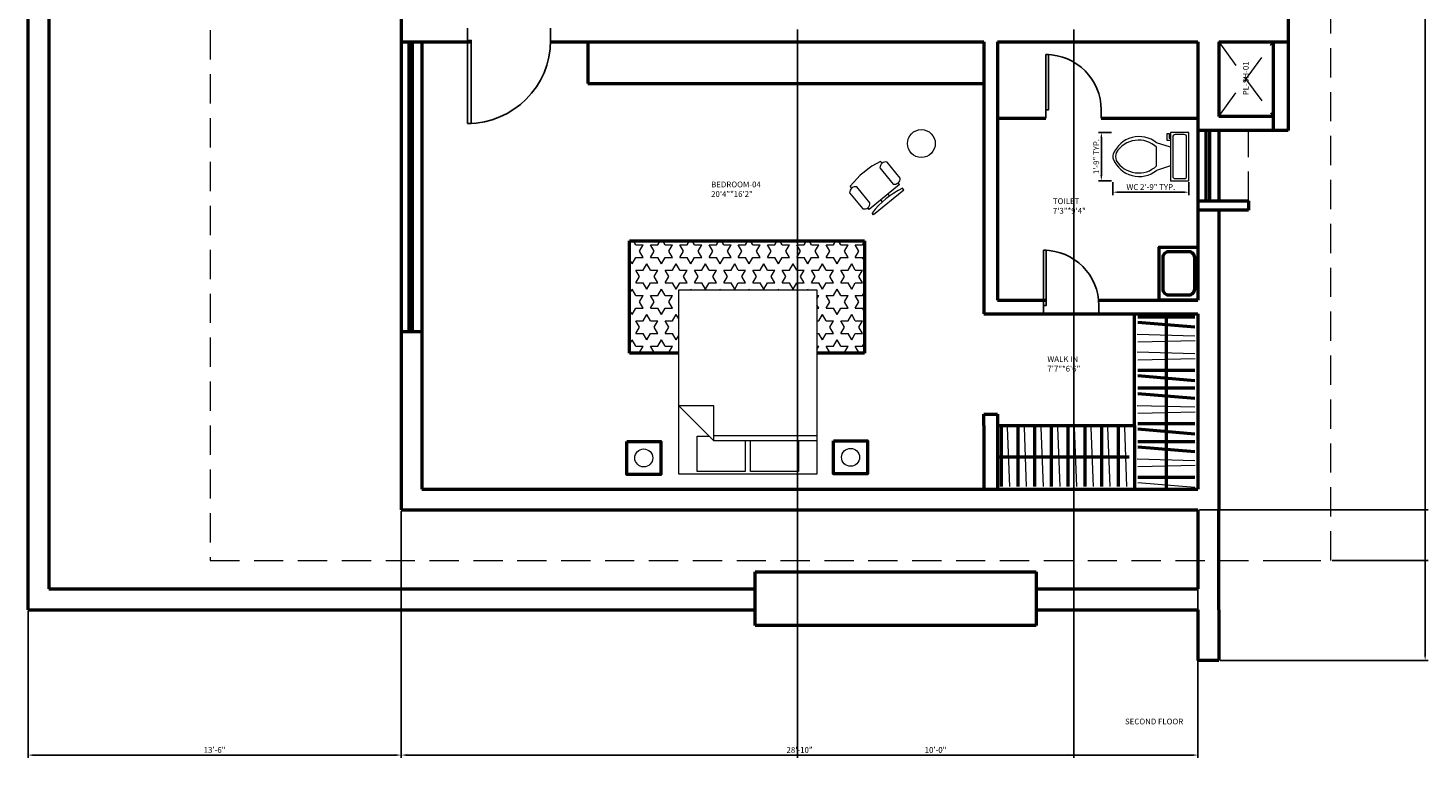
# Model space of a CAD drawing. Units: inches. Extents: x 5312 to 23584, y 2846 to 7447.
# Tile 7 of 12: x 10692 to 11300, y 3035 to 3352. Entities that reach past the tile are written whole.
import ezdxf

# ---------------------------------------------------------------- set-up
doc = ezdxf.new("R2010")
doc.units = ezdxf.units.IN
doc.linetypes.add('DASHED', pattern=[19.05, 12.7, -6.35])
for name, color, linetype, lineweight in [('A-ANNO-DIMS', 2, 'Continuous', 18), ('A-ANNO-TEXT', 3, 'Continuous', 18), ('A-AREA-IDEN', 7, 'Continuous', 18), ('A-DOOR', 4, 'Continuous', 25), ('A-FLOR-FIXT', 9, 'Continuous', 18), ('A-FLOR-OVHD', 8, 'DASHED', 18), ('A-FLOR-PATT', 252, 'Continuous', 13), ('A-FURN', 8, 'Continuous', 18), ('A-WALL', 7, 'Continuous', 50)]:
    doc.layers.add(name, color=color, linetype=linetype, lineweight=lineweight)
doc.styles.get("Standard").update_dxf_attribs({"font": 'arial.ttf'})
doc.dimstyles.new('ISO-25', dxfattribs={"dimtxt": 2.5, "dimasz": 2.5, "dimexe": 1.25, "dimexo": 0.625, "dimtad": 1, "dimlunit": 3, "dimtxsty": 'Standard', "dimcen": 2.5, "dimadec": 0, "dimazin": 0, "dimtfac": 1, "dimtmove": 0, "dimatfit": 3, "dimfxl": 1, "dimarcsym": 0})

# ---------------------------------------------------------------- blocks, each defined once
blk = doc.blocks.new('*U2')
for p, q in [((0, 0), (0, -6)), ((40, 0), (40, -6))]:
    blk.add_line(p, q)
blk.add_lwpolyline([(0, 0), (0, 40), (1.75, 40), (1.75, 0)], close=True)
blk.add_arc((0, 0), 40, 0, 90)
blk = doc.blocks.new('Toilet - top')
for p, q in [((9.5, -6), (9.5, -2)), ((-10, -8.5), (-8, -8.5)), ((-10, -9.5), (-10, -8.5)), ((-7, -9.5), (-10, -9.5)), ((-8, -8.5), (-8, -8)), ((-7, -8), (-7, -9.5)), ((-4, -8), (-6, -14)), ((4, -8), (6, -14)), ((4, -14), (-4, -14))]:
    blk.add_line(p, q)
blk.add_lwpolyline([(10.5, -8), (10.5, 0), (-10.5, 0), (-10.5, -8)], close=True)
for points in [[(-9.5, -2), (-9.5, -6)], [(8.5, -1), (-8.5, -1)], [(-8.5, -7), (8.5, -7)]]:
    blk.add_lwpolyline(points)
for centre, radius, start, end in [((-8.62, -1.88), 0.884, 81.8699, 188.1301), ((-8.62, -6.12), 0.884, 171.8699, 278.1301), ((8.62, -1.88), 0.884, 351.8699, 98.1301), ((8.62, -6.12), 0.884, 261.8699, 8.1301), ((3.52, -21.58), 12.17, 141.46911, 247.97143), ((4.2, -21.82), 11.33, 136.36773, 238.94682), ((-3.52, -21.58), 12.17, 292.02843, 38.53071), ((-4.2, -21.82), 11.33, 301.05301, 43.63209), ((0, -27.88), 4, 245.73182, 294.26817), ((0, -29), 4, 254.86053, 285.13947)]:
    blk.add_arc(centre, radius, start, end)
blk = doc.blocks.new('Bed - Queen')
for p, q in [((0, -80.00003), (0, 0)), ((0, 0), (59.99999, 0)), ((59.99999, 0), (59.99999, -80.00003)), ((7.99999, -1.2), (28.79998, -1.2)), ((7.99999, -14.4), (7.99999, -1.2)), ((28.79998, -1.2), (28.79998, -14.4)), ((31.19999, -1.2), (51.99999, -1.2)), ((31.19999, -14.4), (31.19999, -1.2)), ((51.99999, -1.2), (51.99999, -16.4)), ((0, -14.4), (44.8, -14.4)), ((44.8, -16.8), (0, -16.8)), ((59.99999, -29.6), (44.8, -14.4)), ((44.8, -14.4), (44.8, -29.6)), ((51.99999, -16.4), (46.79936, -16.4)), ((44.8, -29.6), (59.99999, -29.6)), ((59.99999, -80.00003), (0, -80.00003))]:
    blk.add_line(p, q)
blk = doc.blocks.new('Chair - Desk')
for p, q in [((-8.5, 0), (-8.5, -1)), ((-8.5, 0), (8.5, 0)), ((8.5, 0), (8.5, -1)), ((-10.5, -5), (-10.5, -14)), ((-8.5, -3), (-8.5, -4)), ((-8.5, -3), (8.5, -3)), ((-6.5, -14), (-6.5, -5)), ((-2, -3), (-2, -1.9355)), ((2, -1.9576), (2, -3)), ((6.5, -5), (6.5, -14)), ((8.5, -3), (8.5, -4)), ((10.5, -14), (10.5, -5)), ((-8.5, -15), (-8.5, -16)), ((8.5, -15), (8.5, -16))]:
    blk.add_line(p, q)
for centre, radius, start, end in [((-8.5, -6.5), 2.5, 36.8699, 143.1301), ((0, 34.625), 36.625, 256.5803, 283.4197), ((8.5, -6.5), 2.5, 36.8699, 143.1301), ((-8.5, -12.5), 2.5, 216.8699, 323.1301), ((0, 19.625), 36.625, 256.5803, 283.4197), ((8.5, -12.5), 2.5, 216.8699, 323.1301)]:
    blk.add_arc(centre, radius, start, end)
blk = doc.blocks.new('WARDROBE-HANGER')
for p, q in [((0, 3.4), (24.8, 3.4)), ((0, 1.32), (24.99, 0))]:
    blk.add_line(p, q)
blk = doc.blocks.new('*D29')
at = {"layer": 'A-ANNO-DIMS', "color": 0, "lineweight": -2, "transparency": 16777216}
for p, q in [((11162.96, 3285.09), (11162.96, 3279.51)), ((11196.01, 3285.09), (11196.01, 3279.51)), ((11165.46, 3280.76), (11193.51, 3280.76))]:
    blk.add_line(p, q, dxfattribs=at)
at = {"layer": 'A-ANNO-DIMS', "color": 0, "transparency": 16777216}
for points in [[(11165.46, 3281.18), (11165.46, 3280.34), (11162.96, 3280.76)], [(11193.51, 3281.18), (11193.51, 3280.34), (11196.01, 3280.76)]]:
    blk.add_solid(points, dxfattribs=at)
at = {"layer": 'DEFPOINTS', "color": 0, "transparency": 16777216}
for p in [(11162.96, 3285.72), (11196.01, 3285.72), (11196.01, 3280.76)]:
    blk.add_point(p, dxfattribs=at)
at = {"layer": 'A-ANNO-DIMS', "color": 0, "transparency": 16777216, "insert": (11179.49, 3282.68), "char_height": 2.5, "attachment_point": 5}
blk.add_mtext('WC 2\'-9" TYP.', dxfattribs=at)
blk = doc.blocks.new('*D30')
at = {"layer": 'A-ANNO-DIMS', "color": 0, "lineweight": -2, "transparency": 16777216}
for p, q in [((11162.34, 3306.72), (11156.76, 3306.72)), ((11158.01, 3304.22), (11158.01, 3288.22)), ((11162.34, 3285.72), (11156.76, 3285.72))]:
    blk.add_line(p, q, dxfattribs=at)
at = {"layer": 'A-ANNO-DIMS', "color": 0, "transparency": 16777216}
for points in [[(11157.59, 3304.22), (11158.42, 3304.22), (11158.01, 3306.72)], [(11157.59, 3288.22), (11158.42, 3288.22), (11158.01, 3285.72)]]:
    blk.add_solid(points, dxfattribs=at)
at = {"layer": 'DEFPOINTS', "color": 0, "transparency": 16777216}
for p in [(11162.96, 3306.72), (11158.01, 3285.72), (11162.96, 3285.72)]:
    blk.add_point(p, dxfattribs=at)
at = {"layer": 'A-ANNO-DIMS', "color": 0, "transparency": 16777216, "insert": (11156.1, 3296.22), "char_height": 2.5, "attachment_point": 5, "rotation": 90}
blk.add_mtext('1\'-9" TYP.', dxfattribs=at)
blk = doc.blocks.new('*D84')
at = {"layer": 'A-ANNO-DIMS', "color": 0, "lineweight": -2, "transparency": 16777216}
for p, q in [((11209.58, 3832.48), (11299.83, 3832.48)), ((11298.58, 3829.98), (11298.58, 3080.08)), ((11209.58, 3077.58), (11299.83, 3077.58))]:
    blk.add_line(p, q, dxfattribs=at)
at = {"layer": 'A-ANNO-DIMS', "color": 0, "transparency": 16777216}
for points in [[(11298.16, 3829.98), (11298.99, 3829.98), (11298.58, 3832.48)], [(11298.16, 3080.08), (11298.99, 3080.08), (11298.58, 3077.58)]]:
    blk.add_solid(points, dxfattribs=at)
at = {"layer": 'DEFPOINTS', "color": 0, "transparency": 16777216}
for p in [(11208.96, 3832.48), (11208.96, 3077.58), (11298.58, 3077.58)]:
    blk.add_point(p, dxfattribs=at)
at = {"layer": 'A-ANNO-DIMS', "color": 0, "transparency": 16777216, "insert": (11296.68, 3455.03), "char_height": 2.5, "attachment_point": 5, "rotation": 90}
blk.add_mtext('62\'-11"', dxfattribs=at)
blk = doc.blocks.new('*D89')
at = {"layer": 'A-ANNO-DIMS', "color": 0, "lineweight": -2, "transparency": 16777216}
for p, q in [((10853.96, 3142.35), (10853.96, 3035.33)), ((11199.96, 3142.35), (11199.96, 3035.33)), ((10856.46, 3036.58), (11197.46, 3036.58))]:
    blk.add_line(p, q, dxfattribs=at)
at = {"layer": 'A-ANNO-DIMS', "color": 0, "transparency": 16777216}
for points in [[(10856.46, 3037), (10856.46, 3036.17), (10853.96, 3036.58)], [(11197.46, 3037), (11197.46, 3036.17), (11199.96, 3036.58)]]:
    blk.add_solid(points, dxfattribs=at)
at = {"layer": 'DEFPOINTS', "color": 0, "transparency": 16777216}
for p in [(10853.96, 3142.97), (11199.96, 3142.97), (11199.96, 3036.58)]:
    blk.add_point(p, dxfattribs=at)
at = {"layer": 'A-ANNO-DIMS', "color": 0, "transparency": 16777216, "insert": (11026.96, 3038.48), "char_height": 2.5, "attachment_point": 5}
blk.add_mtext('28\'-10"', dxfattribs=at)
blk = doc.blocks.new('*D90')
at = {"layer": 'A-ANNO-DIMS', "color": 0, "lineweight": -2, "transparency": 16777216}
for p, q in [((10853.96, 3142.35), (10853.96, 3035.33)), ((10691.96, 3099.01), (10691.96, 3035.33)), ((10694.46, 3036.58), (10851.46, 3036.58))]:
    blk.add_line(p, q, dxfattribs=at)
at = {"layer": 'A-ANNO-DIMS', "color": 0, "transparency": 16777216}
for points in [[(10694.46, 3037), (10694.46, 3036.17), (10691.96, 3036.58)], [(10851.46, 3037), (10851.46, 3036.17), (10853.96, 3036.58)]]:
    blk.add_solid(points, dxfattribs=at)
at = {"layer": 'DEFPOINTS', "color": 0, "transparency": 16777216}
for p in [(10853.96, 3142.97), (10691.96, 3099.64), (10853.96, 3036.58)]:
    blk.add_point(p, dxfattribs=at)
at = {"layer": 'A-ANNO-DIMS', "color": 0, "transparency": 16777216, "insert": (10772.96, 3038.49), "char_height": 2.5, "attachment_point": 5}
blk.add_mtext('13\'-6"', dxfattribs=at)
blk = doc.blocks.new('*D91')
at = {"layer": 'A-ANNO-DIMS', "color": 0, "lineweight": -2, "transparency": 16777216}
for p, q in [((11200.58, 3706.97), (11299.83, 3706.97)), ((11298.58, 3704.47), (11298.58, 3145.47)), ((11200.58, 3142.97), (11299.83, 3142.97))]:
    blk.add_line(p, q, dxfattribs=at)
at = {"layer": 'A-ANNO-DIMS', "color": 0, "transparency": 16777216}
for points in [[(11298.16, 3704.47), (11298.99, 3704.47), (11298.58, 3706.97)], [(11298.16, 3145.47), (11298.99, 3145.47), (11298.58, 3142.97)]]:
    blk.add_solid(points, dxfattribs=at)
at = {"layer": 'DEFPOINTS', "color": 0, "transparency": 16777216}
for p in [(11199.96, 3706.97), (11199.96, 3142.97), (11298.58, 3142.97)]:
    blk.add_point(p, dxfattribs=at)
at = {"layer": 'A-ANNO-DIMS', "color": 0, "transparency": 16777216, "insert": (11296.68, 3424.97), "char_height": 2.5, "attachment_point": 5, "rotation": 90}
blk.add_mtext('47\'-0"', dxfattribs=at)
blk = doc.blocks.new('*D95')
at = {"layer": 'A-ANNO-DIMS', "color": 0, "lineweight": -2, "transparency": 16777216}
for p, q in [((11258.2, 3751.07), (11299.83, 3751.07)), ((11298.58, 3748.57), (11298.58, 3123.52)), ((11258.2, 3121.02), (11299.83, 3121.02))]:
    blk.add_line(p, q, dxfattribs=at)
at = {"layer": 'A-ANNO-DIMS', "color": 0, "transparency": 16777216}
for points in [[(11298.16, 3748.57), (11298.99, 3748.57), (11298.58, 3751.07)], [(11298.16, 3123.52), (11298.99, 3123.52), (11298.58, 3121.02)]]:
    blk.add_solid(points, dxfattribs=at)
at = {"layer": 'DEFPOINTS', "color": 0, "transparency": 16777216}
for p in [(11257.58, 3751.07), (11257.58, 3121.02), (11298.58, 3121.02)]:
    blk.add_point(p, dxfattribs=at)
at = {"layer": 'A-ANNO-DIMS', "color": 0, "transparency": 16777216, "insert": (11296.68, 3436.04), "char_height": 2.5, "attachment_point": 5, "rotation": 90}
blk.add_mtext('52\'-6"', dxfattribs=at)
blk = doc.blocks.new('*D97')
at = {"layer": 'A-ANNO-DIMS', "color": 0, "lineweight": -2, "transparency": 16777216}
for p, q in [((11026, 3351.35), (11026, 3035.33)), ((11146, 3351.35), (11146, 3035.33)), ((11028.5, 3036.58), (11143.5, 3036.58))]:
    blk.add_line(p, q, dxfattribs=at)
at = {"layer": 'A-ANNO-DIMS', "color": 0, "transparency": 16777216}
for points in [[(11028.5, 3037), (11028.5, 3036.17), (11026, 3036.58)], [(11143.5, 3037), (11143.5, 3036.17), (11146, 3036.58)]]:
    blk.add_solid(points, dxfattribs=at)
at = {"layer": 'DEFPOINTS', "color": 0, "transparency": 16777216}
for p in [(11026, 3351.97), (11146, 3351.97), (11146, 3036.58)]:
    blk.add_point(p, dxfattribs=at)
at = {"layer": 'A-ANNO-DIMS', "color": 0, "transparency": 16777216, "insert": (11086, 3038.48), "char_height": 2.5, "attachment_point": 5}
blk.add_mtext('10\'-0"', dxfattribs=at)

msp = doc.modelspace()

# ---------------------------------------------------------------- hatches: boundary and pattern name
at = {"layer": 'A-FLOR-PATT'}
h = msp.add_hatch(dxfattribs=at)
h.set_pattern_fill('STARS', color=256)
h.set_pattern_definition([(0, (27.571, -223.0893), (0, 5.4992613), [3.175, -3.175]), (60, (27.571, -223.0893), (-4.7625, 2.7496307), [3.175, -3.175]), (120, (29.1586, -220.3397), (-4.7625, -2.7496307), [3.175, -3.175])])
h.paths.add_polyline_path([(11055.106, 3259.675), (10953.169, 3259.675), (10953.169, 3210.954), (10974.489, 3210.954), (10974.489, 3238.461), (11034.489, 3238.461), (11034.489, 3210.954), (11055.106, 3210.954)])

# ---------------------------------------------------------------- linework, layer by layer
at = {"layer": 'A-FLOR-OVHD'}
for p, q in [((10771.06, 3751.067), (10771.06, 3121.017)), ((11257.577, 3121.017), (11257.577, 3751.067)), ((11208.956, 3345.971), (11232.596, 3313.569)), ((11208.956, 3313.569), (11232.596, 3345.971)), ((11221.852, 3276.968), (11221.852, 3307.569)), ((10771.06, 3121.017), (11240.609, 3121.017)), ((11240.609, 3121.017), (11257.577, 3121.017))]:
    msp.add_line(p, q, dxfattribs=at)
at = {"layer": 'A-FURN'}
for p, q in [((11117.157, 3178.678), (11118.144, 3153.125)), ((11124.419, 3178.678), (11125.405, 3153.125)), ((11131.68, 3178.678), (11132.666, 3153.125)), ((11138.941, 3178.678), (11139.927, 3153.125)), ((11146.203, 3178.678), (11147.189, 3153.125)), ((11153.464, 3178.678), (11154.45, 3153.125)), ((11160.725, 3178.678), (11161.711, 3153.125)), ((11167.987, 3178.678), (11168.973, 3153.125)), ((11173.853, 3154.871), (11198.546, 3152.788))]:
    msp.add_line(p, q, dxfattribs=at)
for centre, radius in [((11079.861, 3301.87), 6.038), ((10959.33, 3165.472), 3.898), ((11049.101, 3165.75), 3.898)]:
    msp.add_circle(centre, radius, dxfattribs=at)
at = {"layer": 'A-WALL'}
for p, q in [((10700.956, 3790.971), (10700.956, 3108.64)), ((10853.956, 3706.971), (10853.956, 3142.971)), ((11239.069, 3394.056), (11239.069, 3307.569)), ((10691.956, 3375.201), (10691.956, 3099.64)), ((10853.956, 3345.971), (10884.418, 3345.971)), ((10857.312, 3345.971), (10857.312, 3220.265)), ((10858.699, 3345.971), (10858.699, 3345.971)), ((10858.699, 3345.971), (10858.699, 3220.265)), ((10862.956, 3345.971), (10862.956, 3151.971)), ((10918.838, 3345.971), (11106.956, 3345.971)), ((10934.962, 3345.971), (10934.962, 3327.899)), ((11106.956, 3345.971), (11106.956, 3227.971)), ((11112.956, 3345.971), (11112.956, 3233.971)), ((11112.956, 3345.971), (11199.956, 3345.971)), ((11199.956, 3345.971), (11199.956, 3233.971)), ((11208.956, 3345.971), (11208.956, 3313.569)), ((11208.956, 3345.971), (11239.069, 3345.971)), ((11232.596, 3345.971), (11232.596, 3307.569)), ((10934.962, 3327.899), (11106.956, 3327.899)), ((11232.596, 3313.569), (11208.956, 3313.569)), ((11112.956, 3312.826), (11114.056, 3312.826)), ((11114.056, 3312.826), (11133.935, 3312.826)), ((11157.935, 3312.826), (11199.956, 3312.826)), ((11232.596, 3307.569), (11199.956, 3307.569)), ((11203.397, 3307.569), (11203.397, 3276.968)), ((11204.986, 3307.569), (11204.986, 3307.569)), ((11204.986, 3307.569), (11204.986, 3276.968)), ((11208.956, 3307.569), (11208.956, 3276.968)), ((11239.069, 3307.569), (11232.596, 3307.569)), ((11199.956, 3276.968), (11221.852, 3276.968)), ((11221.852, 3276.968), (11221.852, 3272.989)), ((11221.852, 3272.989), (11199.956, 3272.989)), ((11208.956, 3272.989), (11208.956, 3181.971)), ((10953.169, 3210.954), (10953.169, 3259.675)), ((10953.169, 3259.675), (11055.106, 3259.675)), ((11055.106, 3259.675), (11055.106, 3210.954)), ((11112.956, 3233.971), (11133.99, 3233.971)), ((11156.82, 3233.971), (11199.956, 3233.971)), ((11106.956, 3227.971), (11199.956, 3227.971)), ((11172.44, 3179.625), (11172.44, 3227.971)), ((11199.956, 3227.971), (11199.956, 3151.971)), ((11173.853, 3226.747), (11198.546, 3226.747)), ((11173.853, 3224.407), (11198.546, 3222.324)), ((11186.199, 3227.335), (11186.199, 3152.729)), ((10853.956, 3220.265), (10862.956, 3220.265)), ((10974.489, 3210.954), (10953.169, 3210.954)), ((11055.106, 3210.954), (11034.489, 3210.954)), ((11173.853, 3203.569), (11198.546, 3203.569)), ((11173.853, 3201.228), (11198.546, 3199.146)), ((11173.853, 3195.843), (11198.546, 3195.843)), ((11173.853, 3193.502), (11198.546, 3191.419)), ((11106.956, 3179.625), (11106.956, 3184.528)), ((11106.956, 3184.528), (11112.956, 3184.528)), ((11106.956, 3179.625), (11106.956, 3151.971)), ((11112.956, 3184.528), (11112.956, 3179.625)), ((11112.956, 3179.625), (11172.44, 3179.625)), ((11112.956, 3179.625), (11112.956, 3151.971)), ((11172.44, 3179.625), (11172.44, 3151.971)), ((11173.853, 3180.39), (11198.546, 3180.39)), ((11208.956, 3181.971), (11208.956, 3142.971)), ((11114.472, 3178.678), (11114.472, 3153.125)), ((11121.733, 3178.678), (11121.733, 3153.125)), ((11128.994, 3178.678), (11128.994, 3153.125)), ((11136.255, 3178.678), (11136.255, 3153.125)), ((11143.517, 3178.678), (11143.517, 3153.125)), ((11150.778, 3178.678), (11150.778, 3153.125)), ((11158.039, 3178.678), (11158.039, 3153.125)), ((11165.301, 3178.678), (11165.301, 3153.125)), ((11173.853, 3178.05), (11198.546, 3175.967)), ((11173.853, 3172.664), (11198.546, 3172.664)), ((11173.853, 3170.324), (11198.546, 3168.241)), ((11113.481, 3165.902), (11170.004, 3165.902)), ((11173.853, 3157.212), (11198.546, 3157.212)), ((10862.956, 3151.971), (11199.956, 3151.971)), ((10853.956, 3142.971), (11199.956, 3142.971)), ((11199.956, 3142.971), (11199.956, 3108.64)), ((11208.956, 3099.64), (11208.956, 3142.971)), ((11007.623, 3092.86), (11007.623, 3116.053)), ((11007.623, 3116.053), (11008.103, 3116.053)), ((11008.103, 3116.053), (11129.681, 3116.053)), ((11129.681, 3116.053), (11129.681, 3092.86)), ((10700.956, 3108.64), (11007.623, 3108.64)), ((11129.681, 3108.64), (11199.956, 3108.64)), ((10691.956, 3099.64), (11007.623, 3099.64)), ((11129.681, 3099.64), (11199.956, 3099.64)), ((11199.956, 3099.64), (11199.84, 3077.583)), ((11208.956, 3099.64), (11208.956, 3077.583)), ((11129.681, 3092.86), (11007.623, 3092.86)), ((11199.956, 3077.583), (11199.84, 3077.583)), ((11208.956, 3077.583), (11199.956, 3077.583))]:
    msp.add_line(p, q, dxfattribs=at)
for points in [[(11199.956, 3233.971), (11183.169, 3233.971), (11183.169, 3256.944), (11199.956, 3256.944)], [(10951.973, 3172.582), (10966.687, 3172.582), (10966.687, 3158.362), (10951.973, 3158.362)], [(11041.744, 3172.861), (11056.458, 3172.861), (11056.458, 3158.64), (11041.744, 3158.64)]]:
    msp.add_lwpolyline(points, close=True, dxfattribs=at)
msp.add_lwpolyline([(11187.357, 3255.048), (11195.876, 3255.048, -0.4142136), (11198.376, 3252.548), (11198.376, 3238.572, -0.4142136), (11195.876, 3236.072), (11187.357, 3236.072, -0.4142136), (11184.857, 3238.572), (11184.857, 3252.548, -0.4142136)], format="xyb", close=True, dxfattribs=at)

# ---------------------------------------------------------------- block references
at = {"layer": 'A-DOOR', "xscale": -0.9, "yscale": 0.9, "zscale": 0.9, "rotation": 180}
msp.add_blockref('*U2', (10882.843, 3346.571), dxfattribs=at)
at = {"layer": 'A-DOOR', "xscale": 0.6, "yscale": 0.6, "zscale": 0.6}
for p in [(11133.935, 3316.426), (11132.94, 3231.571)]:
    msp.add_blockref('*U2', p, dxfattribs=at)
at = {"layer": 'A-FLOR-FIXT', "rotation": 270}
msp.add_blockref('Toilet - top', (11196.008, 3296.218), dxfattribs=at)
at = {"layer": 'A-FURN'}
for name, p, rotation in [('Chair - Desk', (11065.705, 3276.326), 219.2765593068386), ('Bed - Queen', (11034.489, 3158.461), 180), ('WARDROBE-HANGER', (11198.594, 3219.665), 181.3996685165029), ('WARDROBE-HANGER', (11198.594, 3211.939), 181.3996685165029), ('WARDROBE-HANGER', (11198.594, 3188.76), 181.3996685165029), ('WARDROBE-HANGER', (11198.594, 3165.581), 181.3996685165029)]:
    msp.add_blockref(name, p, dxfattribs=dict(at, rotation=rotation))

# ---------------------------------------------------------------- texts
at = {"layer": 'A-ANNO-TEXT', "insert": (11219.468, 3322.798), "char_height": 2.5, "attachment_point": 1, "rotation": 90}
msp.add_mtext_dynamic_manual_height_columns('PL-SH-01', width=19.1328, gutter_width=12.5, heights=[0], dxfattribs=at)
at = {"layer": 'A-ANNO-TEXT', "insert": (11168.274, 3052.402), "char_height": 2.5, "attachment_point": 1}
msp.add_mtext_dynamic_manual_height_columns('SECOND FLOOR', width=237.02839, gutter_width=12.5, heights=[0], dxfattribs=at)
at = {"layer": 'A-AREA-IDEN', "char_height": 2.5, "attachment_point": 1}
for s, width, insert in [('BEDROOM-04\\P20\'4"*16\'2"', 66.43672, (10988.569, 3285.367)), ('TOILET\\P7\'3"*9\'4"', 40.66947, (11136.959, 3278.105)), ('WALK IN\\P7\'7"*6\'6"', 42.12235, (11134.562, 3209.618))]:
    msp.add_mtext_dynamic_manual_height_columns(s, width=width, gutter_width=12.5, heights=[0], dxfattribs=dict(at, insert=insert))

# ---------------------------------------------------------------- dimensions: what is measured, and where the dimension line sits
at = {"layer": 'A-ANNO-DIMS'}
for base, p1, p2, picture, middle in [((11298.577, 3077.583), (11208.956, 3832.484), (11208.956, 3077.583), '*D84', (11296.675, 3455.034)), ((11298.5767, 3121.0171), (11257.5767, 3751.0665), (11257.5767, 3121.0171), '*D95', (11296.6753, 3436.0418)), ((11298.577, 3142.971), (11199.956, 3706.971), (11199.956, 3142.971), '*D91', (11296.675, 3424.971))]:
    dim = msp.add_linear_dim(base=base, p1=p1, p2=p2, angle=90, dimstyle='ISO-25', override={"dimdec": 1, "dimlfac": 1, "dimrnd": 0, "dimzin": 1, "dimdsep": 46, "dimlunit": 4, "dimfrac": 2}, dxfattribs=at)
    dim.commit()
    dim.dimension.update_dxf_attribs({"geometry": picture, "text_midpoint": middle})
for base, p1, p2, picture, middle in [((11145.998, 3036.583), (11025.998, 3351.971), (11145.998, 3351.971), '*D97', (11085.998, 3038.484)), ((10853.956, 3036.583), (10691.956, 3099.64), (10853.956, 3142.971), '*D90', (10772.956, 3038.485)), ((11199.956, 3036.583), (10853.956, 3142.971), (11199.956, 3142.971), '*D89', (11026.956, 3038.484))]:
    dim = msp.add_linear_dim(base=base, p1=p1, p2=p2, dimstyle='ISO-25', override={"dimdec": 1, "dimlfac": 1, "dimrnd": 0, "dimzin": 1, "dimdsep": 46, "dimlunit": 4, "dimfrac": 2}, dxfattribs=at)
    dim.commit()
    dim.dimension.update_dxf_attribs({"geometry": picture, "text_midpoint": middle})
dim = msp.add_linear_dim(base=(11158.005, 3285.718), p1=(11162.962, 3306.718), p2=(11162.962, 3285.718), angle=270, text='<> TYP.', dimstyle='ISO-25', override={"dimdec": 1, "dimrnd": 0, "dimzin": 1, "dimlunit": 4, "dimfrac": 2}, dxfattribs=at)
dim.commit()
dim.dimension.update_dxf_attribs({"geometry": '*D30', "text_midpoint": (11156.104, 3296.218)})
dim = msp.add_linear_dim(base=(11196.008, 3280.761), p1=(11162.962, 3285.718), p2=(11196.008, 3285.718), text='WC <> TYP.', dimstyle='ISO-25', override={"dimdec": 1, "dimrnd": 0, "dimzin": 1, "dimlunit": 4, "dimfrac": 2}, dxfattribs=at)
dim.commit()
dim.dimension.update_dxf_attribs({"geometry": '*D29', "text_midpoint": (11179.485, 3282.679)})

doc.saveas('drawing.dxf')
